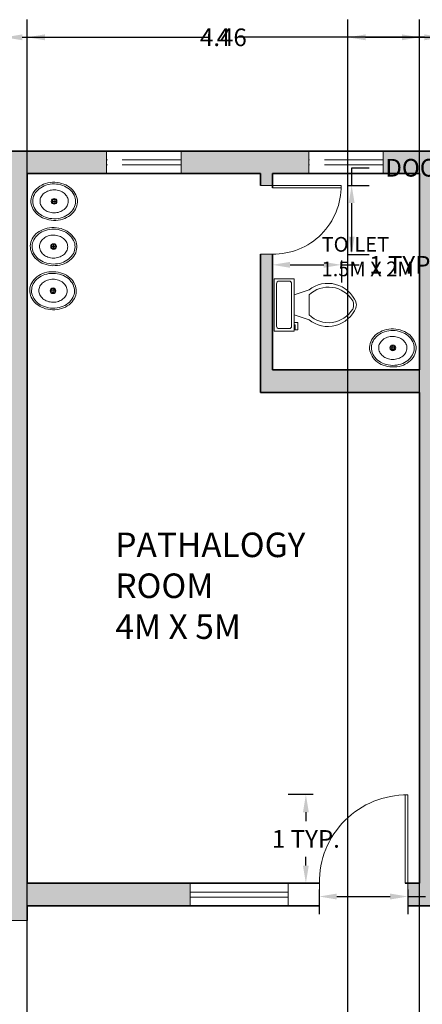
# Model space of a CAD drawing. Units: metres. Extents: x 4298.5 to 4325.2, y 2075 to 2095.8.
# Tile 19 of 35: x 4305.8 to 4309.9, y 2085.8 to 2095.8. Entities that reach past the tile are written whole.
import ezdxf

# ---------------------------------------------------------------- set-up
doc = ezdxf.new("R2010")
doc.units = ezdxf.units.M
doc.linetypes.add('ACAD_ISO02W100', pattern=[15, 12, -3])
for name, color, linetype, lineweight in [('A-ANNO-DIMS', 2, 'Continuous', 18), ('A-AREA-IDEN', 7, 'Continuous', 18), ('A-DOOR', 3, 'Continuous', 18), ('A-FLOR-FIXT', 15, 'Continuous', 18), ('A-GLAZ', 4, 'Continuous', 18), ('A-GLAZ-OVHD', 4, 'ACAD_ISO02W100', 13), ('A-WALL', 7, 'Continuous', 35), ('A-WALL-PATT', 252, 'Continuous', 13)]:
    doc.layers.add(name, color=color, linetype=linetype, lineweight=lineweight)
doc.styles.get("Standard").update_dxf_attribs({"font": 'arial.ttf'})
doc.dimstyles.get("Standard").update_dxf_attribs({"dimtxt": 0.18, "dimasz": 0.18, "dimexe": 0.18, "dimexo": 0.0625, "dimgap": 0.09, "dimtad": 0, "dimtih": 1, "dimtoh": 1, "dimdec": 4, "dimzin": 0, "dimdsep": 46, "dimtxsty": 'Standard', "dimcen": 0.09, "dimadec": 0, "dimazin": 0, "dimtfac": 1, "dimtdec": 4, "dimtofl": 0, "dimtmove": 0, "dimatfit": 3, "dimfxl": 1, "dimtolj": 1, "dimtzin": 0, "dimarcsym": 0})

# ---------------------------------------------------------------- blocks, each defined once
blk = doc.blocks.new('Toilet - top')
for p, q in [((9.5, -6), (9.5, -2)), ((-10, -8.5), (-8, -8.5)), ((-10, -9.5), (-10, -8.5)), ((-7, -9.5), (-10, -9.5)), ((-8, -8.5), (-8, -8)), ((-7, -8), (-7, -9.5)), ((-4, -8), (-6, -14)), ((4, -8), (6, -14)), ((4, -14), (-4, -14))]:
    blk.add_line(p, q)
blk.add_lwpolyline([(10.5, -8), (10.5, 0), (-10.5, 0), (-10.5, -8)], close=True)
for points in [[(-9.5, -2), (-9.5, -6)], [(8.5, -1), (-8.5, -1)], [(-8.5, -7), (8.5, -7)]]:
    blk.add_lwpolyline(points)
for centre, radius, start, end in [((-8.62, -1.88), 0.884, 81.8699, 188.1301), ((8.62, -1.88), 0.884, 351.8699, 98.1301), ((-8.62, -6.12), 0.884, 171.8699, 278.1301), ((8.62, -6.12), 0.884, 261.8699, 8.1301), ((3.52, -21.58), 12.17, 141.4691, 247.9714), ((4.2, -21.82), 11.33, 136.3677, 238.9468), ((-3.52, -21.58), 12.17, 292.0284, 38.5307), ((-4.2, -21.82), 11.33, 301.053, 43.6321), ((0, -27.88), 4, 245.7318, 294.2682), ((0, -29), 4, 254.8605, 285.1395)]:
    blk.add_arc(centre, radius, start, end)
blk = doc.blocks.new('Sink - Oval top')
for p, q in [((-1, 0), (1, 0)), ((0, 1), (0, -1))]:
    blk.add_line(p, q)
for points in [[(-12.23, 0.39, 0.117634), (-11.46, -3.36, 0.104469), (-8.88, -6.8, 0.090016), (-5.08, -9.07, 0.08192), (-0.32, -10.02, 0.08192), (4.49, -9.38, 0.090016), (8.42, -7.36, 0.104469), (11.22, -4.09, 0.117634), (12.23, -0.39, 0.117634), (11.46, 3.36, 0.104469), (8.88, 6.8, 0.090016), (5.08, 9.07, 0.08192), (0.32, 10.02, 0.08192), (-4.49, 9.38, 0.090016), (-8.42, 7.36, 0.104469), (-11.22, 4.09, 0.117634)], [(-11.29, 0.16, 0.118622), (-10.52, -3.25, 0.104678), (-8.07, -6.36, 0.089562), (-4.54, -8.37, 0.081185), (-0.13, -9.15, 0.081185), (4.3, -8.49, 0.089562), (7.89, -6.58, 0.104678), (10.42, -3.55, 0.118622), (11.29, -0.16, 0.118622), (10.52, 3.25, 0.104678), (8.07, 6.36, 0.089562), (4.54, 8.37, 0.081185), (0.13, 9.15, 0.081185), (-4.3, 8.49, 0.089562), (-7.89, 6.58, 0.104678), (-10.42, 3.55, 0.118622)], [(-7.42, 0.08, 0.118283), (-6.91, -2.17, 0.104607), (-5.29, -4.21, 0.089718), (-2.97, -5.53, 0.081436), (-0.07, -6.04, 0.081436), (2.84, -5.59, 0.089718), (5.2, -4.33, 0.104607), (6.86, -2.32, 0.118283), (7.42, -0.08, 0.118283), (6.91, 2.17, 0.104607), (5.29, 4.21, 0.089718), (2.97, 5.53, 0.081436), (0.07, 6.04, 0.081436), (-2.84, 5.59, 0.089718), (-5.2, 4.33, 0.104607), (-6.86, 2.32, 0.118283)]]:
    blk.add_lwpolyline(points, format="xyb", close=True)
for radius in [1.5, 1]:
    blk.add_circle((0, 0), radius)
blk = doc.blocks.new('WIN-1000-GLASS')
for p, q in [((1, 0.05), (0, 0.05)), ((1, 0), (0, 0))]:
    blk.add_line(p, q)
blk = doc.blocks.new('WIN-760-GLASS-HIGH')
at = {"ltscale": 0.05}
for p, q in [((0, 0.76), (0, 0)), ((0.05, 0.76), (0.05, 0))]:
    blk.add_line(p, q, dxfattribs=at)
blk = doc.blocks.new('DOOR-900-LEAF')
for p, q in [((0.9, 0.9), (0, 0.9)), ((0.9, 0.875), (0, 0.875))]:
    blk.add_line(p, q)
blk.add_arc((0.8875, 0.8875), 0.8876, 179.19307, 270.80693)
blk = doc.blocks.new('DOOR-700-LEAF')
for p, q in [((0.675, 0), (0.675, 0.7)), ((0.7, 0), (0.7, 0.7))]:
    blk.add_line(p, q)
blk.add_arc((0.688, 0.012), 0.688, 88.9584, 181.0416)
blk = doc.blocks.new('*D29')
at = {"layer": 'A-ANNO-DIMS', "color": 0, "lineweight": -2, "transparency": 16777216}
for p, q in [((4308.867, 2086.956), (4308.867, 2086.703)), ((4309.047, 2086.883), (4309.591, 2086.883)), ((4309.771, 2086.956), (4309.771, 2086.703)), ((4309.771, 2086.883), (4309.951, 2086.883))]:
    blk.add_line(p, q, dxfattribs=at)
at = {"layer": 'A-ANNO-DIMS', "color": 0, "transparency": 16777216}
for points in [[(4309.047, 2086.913), (4309.047, 2086.853), (4308.867, 2086.883)], [(4309.591, 2086.913), (4309.591, 2086.853), (4309.771, 2086.883)]]:
    blk.add_solid(points, dxfattribs=at)
at = {"layer": 'Defpoints', "color": 0, "transparency": 16777216}
for p in [(4308.867, 2087.018), (4309.771, 2087.018), (4309.771, 2086.883)]:
    blk.add_point(p, dxfattribs=at)
at = {"layer": 'A-ANNO-DIMS', "color": 0, "transparency": 16777216, "insert": (4311.012, 2086.883), "char_height": 0.18, "attachment_point": 5}
blk.add_mtext('\\A1;DOOR D1 1 TYP.', dxfattribs=at)
blk = doc.blocks.new('*D30')
at = {"layer": 'A-ANNO-DIMS', "color": 0, "lineweight": -2, "transparency": 16777216}
for p, q in [((4308.805, 2087.921), (4308.552, 2087.921)), ((4308.732, 2087.741), (4308.732, 2087.65)), ((4308.732, 2087.198), (4308.732, 2087.289)), ((4308.805, 2087.018), (4308.552, 2087.018))]:
    blk.add_line(p, q, dxfattribs=at)
at = {"layer": 'A-ANNO-DIMS', "color": 0, "transparency": 16777216}
for points in [[(4308.702, 2087.741), (4308.762, 2087.741), (4308.732, 2087.921)], [(4308.702, 2087.198), (4308.762, 2087.198), (4308.732, 2087.018)]]:
    blk.add_solid(points, dxfattribs=at)
at = {"layer": 'Defpoints', "color": 0, "transparency": 16777216}
for p in [(4308.867, 2087.921), (4308.732, 2087.018), (4308.867, 2087.018)]:
    blk.add_point(p, dxfattribs=at)
at = {"layer": 'A-ANNO-DIMS', "color": 0, "transparency": 16777216, "insert": (4308.732, 2087.47), "char_height": 0.18, "attachment_point": 5}
blk.add_mtext('\\A1;1 TYP.', dxfattribs=at)
blk = doc.blocks.new('*D33')
at = {"layer": 'A-ANNO-DIMS', "color": 0, "lineweight": -2, "transparency": 16777216}
for p, q in [((4309.199, 2094.128), (4309.199, 2094.308)), ((4309.199, 2094.308), (4309.379, 2094.308)), ((4309.156, 2094.128), (4309.379, 2094.128)), ((4309.199, 2093.605), (4309.199, 2093.948)), ((4309.156, 2093.425), (4309.379, 2093.425))]:
    blk.add_line(p, q, dxfattribs=at)
at = {"layer": 'A-ANNO-DIMS', "color": 0, "transparency": 16777216}
for points in [[(4309.169, 2093.948), (4309.229, 2093.948), (4309.199, 2094.128)], [(4309.169, 2093.605), (4309.229, 2093.605), (4309.199, 2093.425)]]:
    blk.add_solid(points, dxfattribs=at)
at = {"layer": 'Defpoints', "color": 0, "transparency": 16777216}
for p in [(4309.094, 2094.128), (4309.199, 2094.128), (4309.094, 2093.425)]:
    blk.add_point(p, dxfattribs=at)
at = {"layer": 'A-ANNO-DIMS', "color": 0, "transparency": 16777216, "insert": (4310.441, 2094.308), "char_height": 0.18, "attachment_point": 5}
blk.add_mtext('\\A1;DOOR D2 1 TYP.', dxfattribs=at)
blk = doc.blocks.new('*D34')
at = {"layer": 'A-ANNO-DIMS', "color": 0, "lineweight": -2, "transparency": 16777216}
for p, q in [((4308.391, 2093.362), (4308.391, 2093.139)), ((4308.571, 2093.319), (4308.914, 2093.319)), ((4309.094, 2093.362), (4309.094, 2093.139)), ((4309.094, 2093.319), (4309.274, 2093.319))]:
    blk.add_line(p, q, dxfattribs=at)
at = {"layer": 'A-ANNO-DIMS', "color": 0, "transparency": 16777216}
for points in [[(4308.571, 2093.349), (4308.571, 2093.289), (4308.391, 2093.319)], [(4308.914, 2093.349), (4308.914, 2093.289), (4309.094, 2093.319)]]:
    blk.add_solid(points, dxfattribs=at)
at = {"layer": 'Defpoints', "color": 0, "transparency": 16777216}
for p in [(4308.391, 2093.425), (4309.094, 2093.425), (4309.094, 2093.319)]:
    blk.add_point(p, dxfattribs=at)
at = {"layer": 'A-ANNO-DIMS', "color": 0, "transparency": 16777216, "insert": (4309.724, 2093.319), "char_height": 0.18, "attachment_point": 5}
blk.add_mtext('\\A1;1 TYP.', dxfattribs=at)
blk = doc.blocks.new('*D50')
at = {"layer": 'A-ANNO-DIMS', "color": 0, "lineweight": -2, "transparency": 16777216}
for p, q in [((4305.661, 2094.541), (4305.661, 2095.817)), ((4310.121, 2094.541), (4310.121, 2095.817)), ((4305.841, 2095.637), (4307.563, 2095.637)), ((4309.941, 2095.637), (4308.218, 2095.637))]:
    blk.add_line(p, q, dxfattribs=at)
at = {"layer": 'A-ANNO-DIMS', "color": 0, "transparency": 16777216}
for points in [[(4305.841, 2095.667), (4305.841, 2095.607), (4305.661, 2095.637)], [(4309.941, 2095.667), (4309.941, 2095.607), (4310.121, 2095.637)]]:
    blk.add_solid(points, dxfattribs=at)
at = {"layer": 'Defpoints', "color": 0, "transparency": 16777216}
for p in [(4310.121, 2095.637), (4305.661, 2094.478), (4310.121, 2094.478)]:
    blk.add_point(p, dxfattribs=at)
at = {"layer": 'A-ANNO-DIMS', "color": 0, "transparency": 16777216, "insert": (4307.891, 2095.637), "char_height": 0.18, "attachment_point": 5}
blk.add_mtext('\\A1;4.46', dxfattribs=at)
blk = doc.blocks.new('*D53')
at = {"layer": 'A-ANNO-DIMS', "color": 0, "lineweight": -2, "transparency": 16777216}
for p, q in [((4309.161, 2076.391), (4309.161, 2095.817)), ((4316.811, 2076.391), (4316.811, 2095.817)), ((4309.341, 2095.637), (4312.662, 2095.637)), ((4316.631, 2095.637), (4313.309, 2095.637))]:
    blk.add_line(p, q, dxfattribs=at)
at = {"layer": 'A-ANNO-DIMS', "color": 0, "transparency": 16777216}
for points in [[(4309.341, 2095.667), (4309.341, 2095.607), (4309.161, 2095.637)], [(4316.631, 2095.667), (4316.631, 2095.607), (4316.811, 2095.637)]]:
    blk.add_solid(points, dxfattribs=at)
at = {"layer": 'Defpoints', "color": 0, "transparency": 16777216}
for p in [(4316.811, 2095.637), (4309.161, 2076.328), (4316.811, 2076.328)]:
    blk.add_point(p, dxfattribs=at)
at = {"layer": 'A-ANNO-DIMS', "color": 0, "transparency": 16777216, "insert": (4312.986, 2095.637), "char_height": 0.18, "attachment_point": 5}
blk.add_mtext('\\A1;7.65', dxfattribs=at)
blk = doc.blocks.new('*D57')
at = {"layer": 'A-ANNO-DIMS', "color": 0, "lineweight": -2, "transparency": 16777216}
for p, q in [((4305.891, 2085.121), (4305.891, 2095.817)), ((4309.891, 2085.121), (4309.891, 2095.817)), ((4306.071, 2095.637), (4307.738, 2095.637)), ((4309.711, 2095.637), (4308.043, 2095.637))]:
    blk.add_line(p, q, dxfattribs=at)
at = {"layer": 'A-ANNO-DIMS', "color": 0, "transparency": 16777216}
for points in [[(4306.071, 2095.667), (4306.071, 2095.607), (4305.891, 2095.637)], [(4309.711, 2095.667), (4309.711, 2095.607), (4309.891, 2095.637)]]:
    blk.add_solid(points, dxfattribs=at)
at = {"layer": 'Defpoints', "color": 0, "transparency": 16777216}
for p in [(4309.891, 2095.637), (4305.891, 2085.058), (4309.891, 2085.058)]:
    blk.add_point(p, dxfattribs=at)
at = {"layer": 'A-ANNO-DIMS', "color": 0, "transparency": 16777216, "insert": (4307.891, 2095.637), "char_height": 0.18, "attachment_point": 5}
blk.add_mtext('\\A1;4', dxfattribs=at)

msp = doc.modelspace()

# ---------------------------------------------------------------- hatches: boundary and pattern name
at = {"layer": 'A-WALL-PATT'}
h = msp.add_hatch(color=256, dxfattribs=at)
h.dxf.hatch_style = 1
h.paths.add_polyline_path([(4308.7606, 2094.4781), (4308.1606, 2094.4781), (4307.4606, 2094.4781), (4307.4606, 2094.2481), (4308.2706, 2094.2481), (4308.2706, 2094.1281), (4308.3906, 2094.1281), (4308.3906, 2094.2481), (4308.7606, 2094.2481)])
h.paths.add_polyline_path([(4310.1206, 2094.4781), (4309.5206, 2094.4781), (4309.5206, 2094.2481), (4309.8906, 2094.2481), (4309.8906, 2092.2481), (4308.3906, 2092.2481), (4308.3906, 2093.4281), (4308.2706, 2093.4281), (4308.2706, 2092.0181), (4309.8906, 2092.0181), (4309.8906, 2087.0181), (4309.7706, 2087.0181), (4309.7706, 2086.7881), (4309.8906, 2086.7881), (4311.9406, 2086.7881), (4311.9406, 2087.0181), (4310.1206, 2087.0181), (4310.1206, 2089.0181), (4310.2406, 2089.0181), (4310.2406, 2089.1381), (4310.1206, 2089.1381), (4310.1206, 2092.0181), (4310.3078, 2092.0181), (4310.3078, 2092.2481), (4310.1206, 2092.2481)])
h.paths.add_polyline_path([(4311.7406, 2092.2481), (4311.0678, 2092.2481), (4311.0678, 2092.0181), (4311.7406, 2092.0181)], flags=17)
h.paths.add_polyline_path([(4313.1733, 2092.2481), (4312.5006, 2092.2481), (4312.5006, 2092.0181), (4313.1733, 2092.0181)])
h.paths.add_polyline_path([(4314.5378, 2092.2481), (4314.1206, 2092.2481), (4313.9333, 2092.2481), (4313.9333, 2092.0181), (4314.1206, 2092.0181), (4314.1206, 2087.0181), (4314.0006, 2087.0181), (4314.0006, 2086.7881), (4314.1206, 2086.7881), (4315.5718, 2086.7881), (4315.5718, 2087.0181), (4314.3506, 2087.0181), (4314.3506, 2092.0181), (4314.5378, 2092.0181)])
h.paths.add_polyline_path([(4315.9706, 2092.2481), (4315.2978, 2092.2481), (4315.2978, 2092.0181), (4315.9706, 2092.0181)])
h.paths.add_polyline_path([(4317.4033, 2092.2481), (4316.7306, 2092.2481), (4316.7306, 2092.0181), (4317.4033, 2092.0181)])
h.paths.add_polyline_path([(4318.9506, 2092.2481), (4318.3506, 2092.2481), (4318.1633, 2092.2481), (4318.1633, 2092.0181), (4318.3506, 2092.0181), (4318.3506, 2091.8981), (4318.5806, 2091.8981), (4318.5806, 2092.0181), (4318.9506, 2092.0181)])
h.paths.add_polyline_path([(4321.0106, 2092.2481), (4319.7106, 2092.2481), (4319.7106, 2092.0181), (4320.0806, 2092.0181), (4320.0806, 2090.0181), (4318.5806, 2090.0181), (4318.5806, 2091.1981), (4318.3506, 2091.1981), (4318.3506, 2090.0181), (4318.3506, 2087.0181), (4318.2306, 2087.0181), (4318.2306, 2086.7881), (4318.3506, 2086.7881), (4318.3506, 2086.3081), (4318.5806, 2086.3081), (4318.5806, 2089.7881), (4321.7806, 2089.7881), (4321.7806, 2090.0181), (4320.2006, 2090.0181), (4320.2006, 2092.0181), (4321.0106, 2092.0181)])
h.paths.add_polyline_path([(4322.8106, 2092.2481), (4321.7706, 2092.2481), (4321.7706, 2092.0181), (4322.5806, 2092.0181), (4322.5806, 2091.2831), (4322.8106, 2091.2831)])
h.paths.add_polyline_path([(4322.8106, 2090.5231), (4322.5806, 2090.5231), (4322.5806, 2089.7881), (4322.5806, 2089.5254), (4322.8106, 2089.5254), (4322.8106, 2090.0181)])
h.paths.add_polyline_path([(4322.8106, 2088.7654), (4322.5806, 2088.7654), (4322.5806, 2087.6681), (4322.8106, 2087.6681)])
h.paths.add_polyline_path([(4322.8106, 2086.9081), (4322.5806, 2086.9081), (4322.5806, 2085.8107), (4322.8106, 2085.8107)])
h.paths.add_polyline_path([(4322.8106, 2085.0507), (4322.5806, 2085.0507), (4322.5806, 2084.7881), (4318.5806, 2084.7881), (4318.5806, 2085.0581), (4318.5806, 2085.4081), (4318.3506, 2085.4081), (4318.3506, 2084.5581), (4318.3506, 2080.8581), (4318.4706, 2080.8581), (4318.4706, 2082.3281), (4319.2606, 2082.3281), (4319.2606, 2082.5581), (4318.5806, 2082.5581), (4318.5806, 2084.5581), (4320.0806, 2084.5581), (4320.0806, 2083.9381), (4320.3106, 2083.9381), (4320.3106, 2084.5581), (4322.8106, 2084.5581)])
h.paths.add_polyline_path([(4320.3106, 2083.1781), (4320.0806, 2083.1781), (4320.0806, 2082.5581), (4319.9606, 2082.5581), (4319.9606, 2082.3281), (4320.0806, 2082.3281), (4320.0806, 2081.5731), (4320.3106, 2081.5731)], flags=17)
h.paths.add_polyline_path([(4320.3106, 2080.8131), (4320.0806, 2080.8131), (4320.0806, 2080.0581), (4318.4286, 2080.0581), (4318.4286, 2079.8281), (4320.3106, 2079.8281)])
h.paths.add_polyline_path([(4317.3506, 2085.2881), (4316.5718, 2085.2881), (4316.5718, 2085.0581), (4317.3506, 2085.0581)])
h.paths.add_polyline_path([(4315.5718, 2085.2881), (4314.8434, 2085.2881), (4314.8434, 2085.0581), (4315.5718, 2085.0581)])
h.paths.add_polyline_path([(4313.8434, 2085.2881), (4312.9406, 2085.2881), (4312.9406, 2085.0581), (4313.8434, 2085.0581)])
h.paths.add_polyline_path([(4311.9406, 2085.2881), (4311.4406, 2085.2881), (4311.4406, 2085.0581), (4311.9406, 2085.0581)])
h.paths.add_polyline_path([(4317.3306, 2087.0181), (4316.5718, 2087.0181), (4316.5718, 2086.7881), (4317.3306, 2086.7881)])
h.paths.add_polyline_path([(4313.1006, 2089.1381), (4311.1406, 2089.1381), (4311.1406, 2089.0181), (4312.9806, 2089.0181), (4312.9806, 2087.0181), (4312.9406, 2087.0181), (4312.9406, 2086.7881), (4313.1006, 2086.7881), (4313.1006, 2087.0181)])
h.paths.add_polyline_path([(4307.5515, 2087.0181), (4305.8906, 2087.0181), (4305.8906, 2092.2481), (4305.8906, 2094.2481), (4306.7006, 2094.2481), (4306.7006, 2094.4781), (4305.6606, 2094.4781), (4305.6606, 2092.2481), (4305.2906, 2092.2481), (4305.2906, 2092.0181), (4305.6606, 2092.0181), (4305.6606, 2090.0181), (4304.1606, 2090.0181), (4304.1606, 2091.1981), (4304.0406, 2091.1981), (4304.0406, 2089.9081), (4301.5606, 2089.9081), (4301.5606, 2089.7881), (4304.0406, 2089.7881), (4305.6606, 2089.7881), (4305.6606, 2086.6381), (4305.8906, 2086.6381), (4305.8906, 2086.7881), (4307.5515, 2086.7881)])
h.paths.add_polyline_path([(4307.5515, 2085.2881), (4305.8906, 2085.2881), (4305.8906, 2085.4381), (4305.6606, 2085.4381), (4305.6606, 2084.7881), (4305.2906, 2084.7881), (4305.2906, 2084.5581), (4305.6606, 2084.5581), (4305.6606, 2084.02), (4305.8906, 2084.02), (4305.8906, 2084.5581), (4305.8906, 2085.0581), (4307.5515, 2085.0581)])
h.paths.add_polyline_path([(4310.2406, 2085.2881), (4308.5515, 2085.2881), (4308.5515, 2085.0581), (4310.2406, 2085.0581)])
h.paths.add_polyline_path([(4317.4286, 2080.0581), (4316.5718, 2080.0581), (4316.5718, 2079.8281), (4317.4286, 2079.8281)])
h.paths.add_polyline_path([(4315.5718, 2080.0581), (4314.8434, 2080.0581), (4314.8434, 2079.8281), (4315.5718, 2079.8281)])
h.paths.add_polyline_path([(4313.8434, 2080.0581), (4312.9406, 2080.0581), (4312.9406, 2079.8281), (4313.8434, 2079.8281)])
h.paths.add_polyline_path([(4311.9406, 2080.0581), (4311.4406, 2080.0581), (4311.4406, 2079.8281), (4311.9406, 2079.8281)])
h.paths.add_polyline_path([(4310.2406, 2080.0581), (4310.1206, 2080.0581), (4310.1206, 2084.0381), (4309.8906, 2084.0381), (4309.8906, 2080.0581), (4309.1606, 2080.0581), (4309.1606, 2079.8281), (4310.2406, 2079.8281)])
h.paths.add_polyline_path([(4308.1606, 2080.0581), (4307.5106, 2080.0581), (4307.5106, 2080.1781), (4307.3906, 2080.1781), (4307.3906, 2080.0581), (4305.8906, 2080.0581), (4305.8906, 2080.567), (4305.6606, 2080.567), (4305.6606, 2079.8281), (4308.1606, 2079.8281)])
h.paths.add_polyline_path([(4307.5106, 2081.9381), (4309.0906, 2081.9381), (4309.0906, 2082.0581), (4305.8906, 2082.0581), (4305.8906, 2083.26), (4305.6606, 2083.26), (4305.6606, 2081.327), (4305.8906, 2081.327), (4305.8906, 2081.9381), (4307.3906, 2081.9381), (4307.3906, 2080.8781), (4307.5106, 2080.8781)])
h.paths.add_polyline_path([(4304.5306, 2084.7881), (4302.7306, 2084.7881), (4302.7306, 2084.5581), (4304.5306, 2084.5581)])
h.paths.add_polyline_path([(4301.9706, 2084.7881), (4300.6606, 2084.7881), (4300.6606, 2085.0249), (4300.4306, 2085.0249), (4300.4306, 2084.5581), (4301.9706, 2084.5581)])
h.paths.add_polyline_path([(4300.6606, 2086.8843), (4300.4306, 2086.8843), (4300.4306, 2085.7849), (4300.6606, 2085.7849)])
h.paths.add_polyline_path([(4300.6606, 2089.1618), (4300.4306, 2089.1618), (4300.4306, 2087.6443), (4300.6606, 2087.6443)])
h.paths.add_polyline_path([(4300.6606, 2091.0212), (4300.4306, 2091.0212), (4300.4306, 2089.9218), (4300.6606, 2089.9218)])
h.paths.add_polyline_path([(4300.6606, 2092.0181), (4301.9706, 2092.0181), (4301.9706, 2092.2481), (4300.4306, 2092.2481), (4300.4306, 2091.7812), (4300.6606, 2091.7812)])
h.paths.add_polyline_path([(4304.5306, 2092.2481), (4302.7306, 2092.2481), (4302.7306, 2092.0181), (4304.0406, 2092.0181), (4304.0406, 2091.8981), (4304.1606, 2091.8981), (4304.1606, 2092.0181), (4304.5306, 2092.0181)], flags=17)

# ---------------------------------------------------------------- linework, layer by layer
at = {"layer": 'A-DOOR'}
for p, q in [((4308.3906, 2094.1281), (4308.2706, 2094.1281)), ((4308.3906, 2093.4281), (4308.2706, 2093.4281)), ((4308.8706, 2087.0181), (4308.8706, 2086.7881)), ((4309.7706, 2087.0181), (4309.7706, 2086.7881)), ((4305.8906, 2086.6381), (4305.6606, 2086.6381))]:
    msp.add_line(p, q, dxfattribs=at)
at = {"layer": 'A-GLAZ'}
for p, q in [((4306.7006, 2094.2481), (4306.7006, 2094.4781)), ((4307.4606, 2094.2481), (4307.4606, 2094.4781)), ((4308.7606, 2094.2481), (4308.7606, 2094.4781)), ((4309.5206, 2094.2481), (4309.5206, 2094.4781)), ((4307.5515, 2087.0181), (4307.5515, 2086.7881)), ((4308.5515, 2087.0181), (4308.5515, 2086.7881))]:
    msp.add_line(p, q, dxfattribs=at)
at = {"layer": 'A-WALL'}
for p, q in [((4308.3906, 2094.4781), (4305.6606, 2094.4781)), ((4310.1206, 2094.4781), (4308.1606, 2094.4781)), ((4308.2706, 2094.2481), (4305.8906, 2094.2481)), ((4305.8906, 2092.0181), (4305.8906, 2094.2481)), ((4308.2706, 2094.2481), (4308.2706, 2094.1281)), ((4309.8906, 2094.2481), (4308.3906, 2094.2481)), ((4308.3906, 2094.2481), (4308.3906, 2094.1031)), ((4309.8906, 2092.2481), (4309.8906, 2094.2481)), ((4308.2706, 2093.4281), (4308.2706, 2092.0181)), ((4308.3906, 2093.4281), (4308.3906, 2092.2481)), ((4305.8906, 2092.2481), (4305.8906, 2087.0181)), ((4309.8906, 2092.2481), (4308.3906, 2092.2481)), ((4305.8906, 2092.0181), (4305.8906, 2087.0181)), ((4309.8906, 2092.0181), (4308.2706, 2092.0181)), ((4309.8906, 2092.0181), (4309.8906, 2087.0181)), ((4305.8906, 2087.0181), (4308.8706, 2087.0181)), ((4309.7456, 2087.0181), (4309.8906, 2087.0181)), ((4305.8906, 2086.7881), (4308.8706, 2086.7881)), ((4305.8906, 2086.7881), (4305.8906, 2086.6381)), ((4309.7706, 2086.7881), (4309.8906, 2086.7881)), ((4309.8906, 2086.7881), (4313.1006, 2086.7881))]:
    msp.add_line(p, q, dxfattribs=at)

# ---------------------------------------------------------------- block references
at = {"layer": 'A-DOOR', "extrusion": (0, 0, -1), "zscale": -1, "rotation": 90.00000000008784}
msp.add_blockref('DOOR-700-LEAF', (-4308.3906, 2093.428), dxfattribs=at)
at = {"layer": 'A-DOOR', "rotation": 270.0000000000276}
msp.add_blockref('DOOR-900-LEAF', (4308.8706, 2087.9181), dxfattribs=at)
at = {"layer": 'A-FLOR-FIXT', "xscale": 0.0193818050953029, "yscale": 0.0193818050953029, "zscale": 0.0193818050953029}
for p in [(4306.1657, 2093.9659), (4306.1599, 2093.5046), (4306.1541, 2093.055), (4309.6185, 2092.4723)]:
    msp.add_blockref('Sink - Oval top', p, dxfattribs=at)
at = {"layer": 'A-FLOR-FIXT', "xscale": 0.0254, "yscale": 0.0254, "zscale": 0.0254, "rotation": 90.00015040587188}
msp.add_blockref('Toilet - top', (4308.4084, 2092.9107), dxfattribs=at)
at = {"layer": 'A-GLAZ'}
msp.add_blockref('WIN-1000-GLASS', (4307.5515, 2086.8781), dxfattribs=at)
at = {"layer": 'A-GLAZ-OVHD'}
for p, rotation in [((4306.7006, 2094.3881), 270.0000000000593), ((4308.7606, 2094.3881), 270.0000000000683)]:
    msp.add_blockref('WIN-760-GLASS-HIGH', p, dxfattribs=dict(at, rotation=rotation))

# ---------------------------------------------------------------- texts
at = {"layer": 'A-AREA-IDEN', "attachment_point": 1}
for s, insert, char_height in [('TOILET\\P1.5M X 2M', (4308.8923, 2093.6028), 0.15), ('PATHALOGY ROOM\\P4M X 5M', (4306.7898, 2090.5911), 0.25)]:
    msp.add_mtext_dynamic_manual_height_columns(s, width=2.22034, gutter_width=12.5, heights=[0], dxfattribs=dict(at, insert=insert, char_height=char_height))

# ---------------------------------------------------------------- dimensions: what is measured, and where the dimension line sits
at = {"layer": 'A-ANNO-DIMS'}
for base, p1, p2, override, picture, middle in [((4310.1206, 2095.6366), (4305.6606, 2094.4781), (4310.1206, 2094.4781), {"dimdec": 2, "dimlfac": 1, "dimrnd": 0, "dimzin": 0, "dimdsep": 46, "dimlunit": 2}, '*D50', (4307.8906, 2095.6366)), ((4309.8906, 2095.6366), (4305.8906, 2085.0581), (4309.8906, 2085.0581), {"dimdec": 0, "dimlfac": 1, "dimrnd": 0, "dimzin": 0, "dimdsep": 46, "dimlunit": 2}, '*D57', (4307.8906, 2095.6366)), ((4316.8106, 2095.6366), (4309.1606, 2076.3281), (4316.8106, 2076.3281), {"dimdec": 2, "dimlfac": 1, "dimrnd": 0, "dimzin": 0, "dimdsep": 46, "dimlunit": 2}, '*D53', (4312.9856, 2095.6366))]:
    dim = msp.add_linear_dim(base=base, p1=p1, p2=p2, dimstyle='Standard', override=override, dxfattribs=at)
    dim.commit()
    dim.dimension.update_dxf_attribs({"geometry": picture, "text_midpoint": middle})
for base, p1, p2, angle, text, picture, middle in [((4309.1995, 2094.1281), (4309.094, 2093.4247), (4309.094, 2094.1281), 90, 'DOOR D2 <> TYP.', '*D33', (4310.4409, 2094.3081)), ((4308.7317, 2087.0181), (4308.8672, 2087.9214), (4308.8672, 2087.0181), 270, '<> TYP.', '*D30', (4308.7317, 2087.4697)), ((4309.7706, 2086.8825), (4308.8672, 2087.0181), (4309.7706, 2087.0181), 0, 'DOOR D1 <> TYP.', '*D29', (4311.012, 2086.8825))]:
    dim = msp.add_linear_dim(base=base, p1=p1, p2=p2, angle=angle, text=text, dimstyle='Standard', override={"dimdec": 0, "dimlfac": 1, "dimrnd": 0, "dimzin": 0, "dimdsep": 46, "dimlunit": 2}, dxfattribs=at)
    dim.commit()
    dim.dimension.update_dxf_attribs({"geometry": picture, "text_midpoint": middle})
dim = msp.add_linear_dim(base=(4309.094, 2093.3192), p1=(4308.3906, 2093.4247), p2=(4309.094, 2093.4247), text='<> TYP.', dimstyle='Standard', override={"dimdec": 0, "dimlfac": 1, "dimrnd": 0, "dimzin": 0, "dimdsep": 46, "dimlunit": 2}, dxfattribs=at)
dim.commit()
dim.dimension.update_dxf_attribs({"geometry": '*D34', "text_midpoint": (4309.7237, 2093.3192)})

doc.saveas('drawing.dxf')
